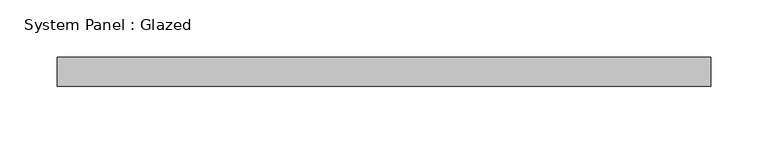
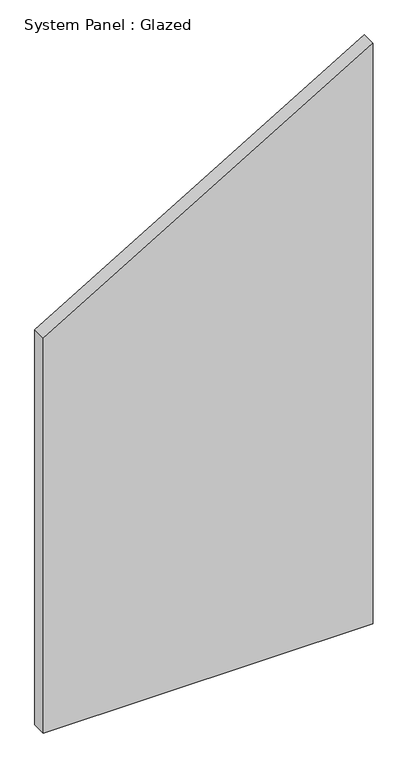
"""IFC4 building model written with IfcOpenShell, lengths in millimetres: plate geometry, System Panel : Glazed."""

from ifc_helpers import new_model, si_unit, frame, origin, place, context, project, spatial, polyline, outline, extrude, source, transform, mapped, element, save


def system_panel_glazed_65593f79(model_context):
    return source(origin(), model_context, "Body", "SweptSolid", [
        extrude(outline(polyline([(0.0, -285.75), (0.0, 285.75), (1062.6231736, 285.75), (722.9554653, -285.75), (0.0, -285.75)])), frame((0.0, 19.05, 0.0), z_axis=(0.0, 1.0, 0.0), x_axis=(0.0, 0.0, 1.0)), (0.0, 0.0, 1.0), 25.4),
    ])


if __name__ == "__main__":
    model = new_model("IFC4")
    model_context = context("Model", 3, world=origin())
    ifc_project = project(units=[si_unit("LENGTHUNIT", "METRE", prefix="MILLI")], contexts=[model_context])
    site = spatial("IfcSite", under=ifc_project)
    building = spatial("IfcBuilding", under=site)
    placement = place(None, origin())
    system_panel_glazed_shape = system_panel_glazed_65593f79(model_context)
    element("IfcPlate", 1, ObjectType="System Panel : Glazed", at=placement, inside=building, context=model_context, shape_type="MappedRepresentation", body=[
        mapped(system_panel_glazed_shape, transform((0.0, 0.0, 0.0), x_axis=(1.0, 0.0, 0.0), y_axis=(0.0, 1.0, 0.0), z_axis=(0.0, 0.0, 1.0))),
    ])
    save(model, "model.ifc")

# Revit data of these elements
# Type "System Panel : Glazed"
#   Construction Type Id = "GSP4R"
#   Analytic Construction = "1/8 in Pilkington single glazing"
#   Visual Light Transmittance = 0.9
#   Solar Heat Gain Coefficient = 0.86
#   Heat Transfer Coefficient (U) = 1.18115 BTU/(h·ft²·°F)
#   Define Thermal Properties by = 1
# Element 1 (IfcPlate, "System Panel : Glazed")
#   Materials on its faces: "Glass"
# Materials
#   "Glass": class "Glass", colour RGB 0 128 192, transparency 0.75, Description = "Soda Lime Glass", Cost = 0
